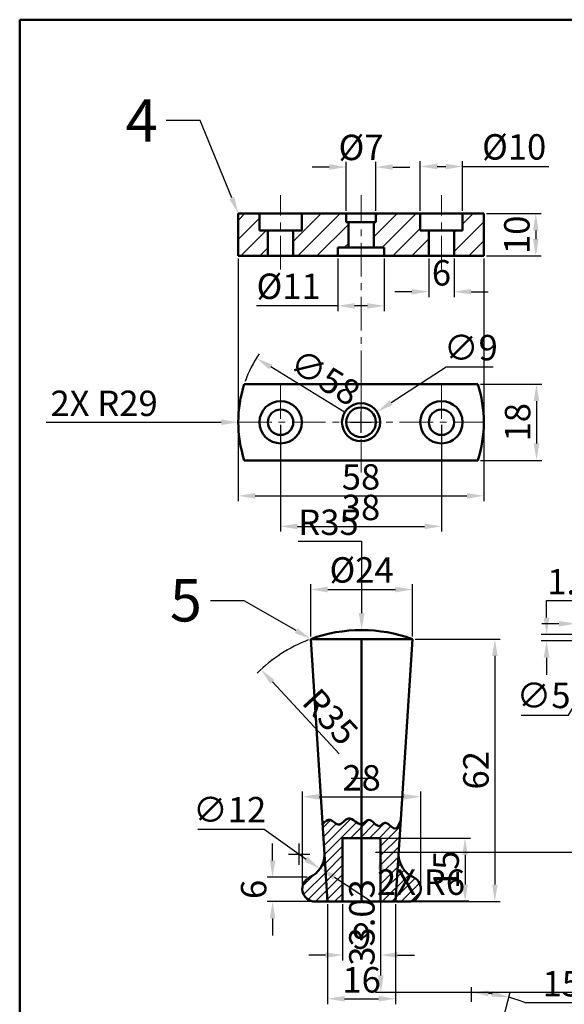
# Model space of a CAD drawing. Units: millimetres. Extents: x 1145 to 1687, y 12 to 400.
# Tile 2 of 6: x 1145 to 1274, y 168 to 400. Entities that reach past the tile are written whole.
import ezdxf
from ezdxf import colors
from ezdxf.entities.mleader import LeaderData, LeaderLine
from ezdxf.math import Vec2, Vec3

# ---------------------------------------------------------------- set-up
doc = ezdxf.new("R2010")
doc.units = ezdxf.units.MM
doc.header["$LTSCALE"] = 0.5
doc.linetypes.add('CENTER', pattern=[50.8, 31.75, -6.35, 6.35, -6.35])
for name, color, linetype, lineweight in [('M-CNTR', 1, 'CENTER', 18), ('M-DIMS', 2, 'Continuous', 25), ('M-HATC', 8, 'Continuous', 18), ('M-OUTL', 7, 'Continuous', 50), ('M-TEXT', 3, 'Continuous', 25)]:
    doc.layers.add(name, color=color, linetype=linetype, lineweight=lineweight)
doc.styles.get("Standard").update_dxf_attribs({"font": 'arial.ttf'})
doc.dimstyles.new('ISO-25', dxfattribs={"dimtxt": 6, "dimasz": 4, "dimexe": 1.25, "dimexo": 0.625, "dimtad": 1, "dimtoh": 1, "dimdec": 0, "dimtxsty": 'Standard', "dimcen": 2.5, "dimadec": 0, "dimazin": 0, "dimtfac": 1, "dimtdec": 0, "dimtofl": 0, "dimtmove": 0, "dimatfit": 3, "dimfxl": 1, "dimarcsym": 0})

# ---------------------------------------------------------------- blocks, each defined once
blk = doc.blocks.new('*D1')
at = {"layer": 'Defpoints', "color": 0, "ltscale": 0.5, "transparency": 16777216}
for p in [(1229.46, 365.34), (1222.46, 354.33), (1229.46, 354.33)]:
    blk.add_point(p, dxfattribs=at)
at = {"layer": 'M-DIMS', "color": 0, "lineweight": -2, "ltscale": 0.5, "transparency": 16777216}
for p, q in [((1218.46, 365.34), (1214.46, 365.34)), ((1222.46, 354.96), (1222.46, 366.59)), ((1229.46, 354.96), (1229.46, 366.59)), ((1233.46, 365.34), (1237.46, 365.34))]:
    blk.add_line(p, q, dxfattribs=at)
at = {"layer": 'M-DIMS', "color": 0, "ltscale": 0.5, "transparency": 16777216}
for points in [[(1218.46, 366), (1218.46, 364.67), (1222.46, 365.34)], [(1233.46, 366), (1233.46, 364.67), (1229.46, 365.34)]]:
    blk.add_solid(points, dxfattribs=at)
at = {"layer": 'M-DIMS', "color": 0, "ltscale": 0.5, "transparency": 16777216, "insert": (1225.96, 369.19), "char_height": 6, "attachment_point": 5}
blk.add_mtext('%%C7', dxfattribs=at)
blk = doc.blocks.new('*D2')
at = {"layer": 'Defpoints', "color": 0, "ltscale": 0.5, "transparency": 16777216}
for p in [(1249.96, 365.46), (1239.96, 354.33), (1249.96, 354.33)]:
    blk.add_point(p, dxfattribs=at)
at = {"layer": 'M-DIMS', "color": 0, "lineweight": -2, "ltscale": 0.5, "transparency": 16777216}
for p, q in [((1239.96, 354.96), (1239.96, 366.71)), ((1243.96, 365.46), (1245.96, 365.46)), ((1249.96, 354.96), (1249.96, 366.71)), ((1249.96, 365.46), (1270.32, 365.46))]:
    blk.add_line(p, q, dxfattribs=at)
at = {"layer": 'M-DIMS', "color": 0, "ltscale": 0.5, "transparency": 16777216}
for points in [[(1243.96, 366.13), (1243.96, 364.8), (1239.96, 365.46)], [(1245.96, 366.13), (1245.96, 364.8), (1249.96, 365.46)]]:
    blk.add_solid(points, dxfattribs=at)
at = {"layer": 'M-DIMS', "color": 0, "ltscale": 0.5, "transparency": 16777216, "insert": (1262.14, 369.32), "char_height": 6, "attachment_point": 5}
blk.add_mtext('%%C10', dxfattribs=at)
blk = doc.blocks.new('*D3')
at = {"layer": 'Defpoints', "color": 0, "ltscale": 0.5, "transparency": 16777216}
for p in [(1254.96, 354.33), (1254.96, 344.33), (1267.24, 344.33)]:
    blk.add_point(p, dxfattribs=at)
at = {"layer": 'M-DIMS', "color": 0, "lineweight": -2, "ltscale": 0.5, "transparency": 16777216}
for p, q in [((1255.59, 354.33), (1268.49, 354.33)), ((1267.24, 350.33), (1267.24, 348.33)), ((1255.59, 344.33), (1268.49, 344.33))]:
    blk.add_line(p, q, dxfattribs=at)
at = {"layer": 'M-DIMS', "color": 0, "ltscale": 0.5, "transparency": 16777216}
for points in [[(1266.58, 350.33), (1267.91, 350.33), (1267.24, 354.33)], [(1266.58, 348.33), (1267.91, 348.33), (1267.24, 344.33)]]:
    blk.add_solid(points, dxfattribs=at)
at = {"layer": 'M-DIMS', "color": 0, "ltscale": 0.5, "transparency": 16777216, "insert": (1263.55, 349.33), "char_height": 6, "attachment_point": 5, "rotation": 90}
blk.add_mtext('10', dxfattribs=at)
blk = doc.blocks.new('*D4')
at = {"layer": 'Defpoints', "color": 0, "ltscale": 0.5, "transparency": 16777216}
for p in [(1241.96, 344.33), (1247.96, 344.33), (1247.96, 335.89)]:
    blk.add_point(p, dxfattribs=at)
at = {"layer": 'M-DIMS', "color": 0, "lineweight": -2, "ltscale": 0.5, "transparency": 16777216}
for p, q in [((1241.96, 343.71), (1241.96, 334.64)), ((1247.96, 343.71), (1247.96, 334.64)), ((1237.96, 335.89), (1233.96, 335.89)), ((1251.96, 335.89), (1255.96, 335.89))]:
    blk.add_line(p, q, dxfattribs=at)
at = {"layer": 'M-DIMS', "color": 0, "ltscale": 0.5, "transparency": 16777216}
for points in [[(1237.96, 336.55), (1237.96, 335.22), (1241.96, 335.89)], [(1251.96, 336.55), (1251.96, 335.22), (1247.96, 335.89)]]:
    blk.add_solid(points, dxfattribs=at)
at = {"layer": 'M-DIMS', "color": 0, "ltscale": 0.5, "transparency": 16777216, "insert": (1244.96, 339.58), "char_height": 6, "attachment_point": 5}
blk.add_mtext('6', dxfattribs=at)
blk = doc.blocks.new('*D5')
at = {"layer": 'Defpoints', "color": 0, "ltscale": 0.5, "transparency": 16777216}
for p in [(1220.46, 344.33), (1231.46, 344.33), (1231.46, 332.54)]:
    blk.add_point(p, dxfattribs=at)
at = {"layer": 'M-DIMS', "color": 0, "lineweight": -2, "ltscale": 0.5, "transparency": 16777216}
for p, q in [((1220.46, 343.71), (1220.46, 331.29)), ((1231.46, 343.71), (1231.46, 331.29)), ((1220.46, 332.54), (1201.25, 332.54)), ((1227.46, 332.54), (1224.46, 332.54))]:
    blk.add_line(p, q, dxfattribs=at)
at = {"layer": 'M-DIMS', "color": 0, "ltscale": 0.5, "transparency": 16777216}
for points in [[(1224.46, 333.21), (1224.46, 331.87), (1220.46, 332.54)], [(1227.46, 333.21), (1227.46, 331.87), (1231.46, 332.54)]]:
    blk.add_solid(points, dxfattribs=at)
at = {"layer": 'M-DIMS', "color": 0, "ltscale": 0.5, "transparency": 16777216, "insert": (1208.86, 336.4), "char_height": 6, "attachment_point": 5}
blk.add_mtext('%%C11', dxfattribs=at)
blk = doc.blocks.new('*D6')
at = {"layer": 'Defpoints', "color": 0, "ltscale": 0.5, "transparency": 16777216}
for p in [(1206.96, 305.06), (1244.96, 305.06), (1244.96, 280.47)]:
    blk.add_point(p, dxfattribs=at)
at = {"layer": 'M-DIMS', "color": 0, "lineweight": -2, "ltscale": 0.5, "transparency": 16777216}
for p, q in [((1206.96, 304.44), (1206.96, 279.22)), ((1244.96, 304.44), (1244.96, 279.22)), ((1210.96, 280.47), (1240.96, 280.47))]:
    blk.add_line(p, q, dxfattribs=at)
at = {"layer": 'M-DIMS', "color": 0, "ltscale": 0.5, "transparency": 16777216}
for points in [[(1210.96, 281.14), (1210.96, 279.8), (1206.96, 280.47)], [(1240.96, 281.14), (1240.96, 279.8), (1244.96, 280.47)]]:
    blk.add_solid(points, dxfattribs=at)
at = {"layer": 'M-DIMS', "color": 0, "ltscale": 0.5, "transparency": 16777216, "insert": (1225.96, 284.16), "char_height": 6, "attachment_point": 5}
blk.add_mtext('38', dxfattribs=at)
blk = doc.blocks.new('*D7')
at = {"layer": 'Defpoints', "color": 0, "ltscale": 0.5, "transparency": 16777216}
for p in [(1253.53, 314.06), (1253.53, 296.06), (1267.41, 296.06)]:
    blk.add_point(p, dxfattribs=at)
at = {"layer": 'M-DIMS', "color": 0, "lineweight": -2, "ltscale": 0.5, "transparency": 16777216}
for p, q in [((1254.16, 314.06), (1268.66, 314.06)), ((1267.41, 310.06), (1267.41, 300.06)), ((1254.16, 296.06), (1268.66, 296.06))]:
    blk.add_line(p, q, dxfattribs=at)
at = {"layer": 'M-DIMS', "color": 0, "ltscale": 0.5, "transparency": 16777216}
for points in [[(1266.74, 310.06), (1268.07, 310.06), (1267.41, 314.06)], [(1266.74, 300.06), (1268.07, 300.06), (1267.41, 296.06)]]:
    blk.add_solid(points, dxfattribs=at)
at = {"layer": 'M-DIMS', "color": 0, "ltscale": 0.5, "transparency": 16777216, "insert": (1263.72, 305.06), "char_height": 6, "attachment_point": 5, "rotation": 90}
blk.add_mtext('18', dxfattribs=at)
blk = doc.blocks.new('*D8')
at = {"layer": 'Defpoints', "color": 0, "ltscale": 0.5, "transparency": 16777216}
for p in [(1229.74, 307.51), (1222.19, 302.62)]:
    blk.add_point(p, dxfattribs=at)
at = {"layer": 'M-DIMS', "color": 0, "lineweight": -2, "ltscale": 0.5, "transparency": 16777216}
for p, q in [((1246.05, 318.06), (1233.1, 309.68)), ((1257.14, 318.06), (1246.05, 318.06)), ((1225.96, 302.56), (1225.96, 307.56)), ((1223.46, 305.06), (1228.46, 305.06))]:
    blk.add_line(p, q, dxfattribs=at)
at = {"layer": 'M-DIMS', "color": 0, "ltscale": 0.5, "transparency": 16777216}
blk.add_solid([(1232.74, 310.24), (1233.46, 309.12), (1229.74, 307.51)], dxfattribs=at)
at = {"layer": 'M-DIMS', "color": 0, "ltscale": 0.5, "transparency": 16777216, "insert": (1251.91, 321.91), "char_height": 6, "attachment_point": 5}
blk.add_mtext('∅9', dxfattribs=at)
blk = doc.blocks.new('*D26')
at = {"layer": 'Defpoints', "color": 0, "ltscale": 0.5, "transparency": 16777216}
for p in [(1221.6, 191.85), (1230.6, 191.85), (1230.6, 179.21)]:
    blk.add_point(p, dxfattribs=at)
at = {"layer": 'M-DIMS', "color": 0, "lineweight": -2, "ltscale": 0.5, "transparency": 16777216}
for p, q in [((1221.6, 191.22), (1221.6, 177.96)), ((1230.6, 191.22), (1230.6, 177.96)), ((1217.6, 179.21), (1213.6, 179.21)), ((1234.6, 179.21), (1238.6, 179.21))]:
    blk.add_line(p, q, dxfattribs=at)
at = {"layer": 'M-DIMS', "color": 0, "ltscale": 0.5, "transparency": 16777216}
for points in [[(1217.6, 179.87), (1217.6, 178.54), (1221.6, 179.21)], [(1234.6, 179.87), (1234.6, 178.54), (1230.6, 179.21)]]:
    blk.add_solid(points, dxfattribs=at)
at = {"layer": 'M-DIMS', "color": 0, "ltscale": 0.5, "transparency": 16777216, "insert": (1226.1, 182.9), "char_height": 6, "attachment_point": 5}
blk.add_mtext('9', dxfattribs=at)
blk = doc.blocks.new('*D27')
at = {"layer": 'Defpoints', "color": 0, "ltscale": 0.5, "transparency": 16777216}
for p in [(1218.07, 191.85), (1234.12, 191.85), (1234.12, 168.89)]:
    blk.add_point(p, dxfattribs=at)
at = {"layer": 'M-DIMS', "color": 0, "lineweight": -2, "ltscale": 0.5, "transparency": 16777216}
for p, q in [((1218.07, 191.22), (1218.07, 167.64)), ((1234.12, 191.22), (1234.12, 167.64)), ((1222.07, 168.89), (1230.12, 168.89))]:
    blk.add_line(p, q, dxfattribs=at)
at = {"layer": 'M-DIMS', "color": 0, "ltscale": 0.5, "transparency": 16777216}
for points in [[(1222.07, 169.55), (1222.07, 168.22), (1218.07, 168.89)], [(1230.12, 169.55), (1230.12, 168.22), (1234.12, 168.89)]]:
    blk.add_solid(points, dxfattribs=at)
at = {"layer": 'M-DIMS', "color": 0, "ltscale": 0.5, "transparency": 16777216, "insert": (1226.1, 172.58), "char_height": 6, "attachment_point": 5}
blk.add_mtext('16', dxfattribs=at)
blk = doc.blocks.new('*D28')
at = {"layer": 'Defpoints', "color": 0, "ltscale": 0.5, "transparency": 16777216}
for p in [(1238.1, 253.85), (1234.12, 191.85), (1257.57, 191.85)]:
    blk.add_point(p, dxfattribs=at)
at = {"layer": 'M-DIMS', "color": 0, "lineweight": -2, "ltscale": 0.5, "transparency": 16777216}
for p, q in [((1238.72, 253.85), (1258.82, 253.85)), ((1257.57, 249.85), (1257.57, 195.85)), ((1234.75, 191.85), (1258.82, 191.85))]:
    blk.add_line(p, q, dxfattribs=at)
at = {"layer": 'M-DIMS', "color": 0, "ltscale": 0.5, "transparency": 16777216}
for points in [[(1256.91, 249.85), (1258.24, 249.85), (1257.57, 253.85)], [(1256.91, 195.85), (1258.24, 195.85), (1257.57, 191.85)]]:
    blk.add_solid(points, dxfattribs=at)
at = {"layer": 'M-DIMS', "color": 0, "ltscale": 0.5, "transparency": 16777216, "insert": (1253.88, 222.85), "char_height": 6, "attachment_point": 5, "rotation": 90}
blk.add_mtext('62', dxfattribs=at)
blk = doc.blocks.new('*D29')
at = {"layer": 'Defpoints', "color": 0, "ltscale": 0.5, "transparency": 16777216}
for p in [(1226.1, 206.85), (1226.1, 191.85), (1250.54, 191.85)]:
    blk.add_point(p, dxfattribs=at)
at = {"layer": 'M-DIMS', "color": 0, "lineweight": -2, "ltscale": 0.5, "transparency": 16777216}
for p, q in [((1226.72, 206.85), (1251.79, 206.85)), ((1250.54, 202.85), (1250.54, 195.85)), ((1226.72, 191.85), (1251.79, 191.85))]:
    blk.add_line(p, q, dxfattribs=at)
at = {"layer": 'M-DIMS', "color": 0, "ltscale": 0.5, "transparency": 16777216}
for points in [[(1249.87, 202.85), (1251.2, 202.85), (1250.54, 206.85)], [(1249.87, 195.85), (1251.2, 195.85), (1250.54, 191.85)]]:
    blk.add_solid(points, dxfattribs=at)
at = {"layer": 'M-DIMS', "color": 0, "ltscale": 0.5, "transparency": 16777216, "insert": (1246.85, 199.35), "char_height": 6, "attachment_point": 5, "rotation": 90}
blk.add_mtext('15', dxfattribs=at)
blk = doc.blocks.new('*D30')
at = {"layer": 'Defpoints', "color": 0, "ltscale": 0.5, "transparency": 16777216}
for p in [(1205.07, 197.58), (1213.85, 197.58), (1215.1, 191.85)]:
    blk.add_point(p, dxfattribs=at)
at = {"layer": 'M-DIMS', "color": 0, "lineweight": -2, "ltscale": 0.5, "transparency": 16777216}
for p, q in [((1205.07, 201.58), (1205.07, 205.58)), ((1213.23, 197.58), (1203.82, 197.58)), ((1214.47, 191.85), (1203.82, 191.85)), ((1205.07, 187.85), (1205.07, 183.85))]:
    blk.add_line(p, q, dxfattribs=at)
at = {"layer": 'M-DIMS', "color": 0, "ltscale": 0.5, "transparency": 16777216}
for points in [[(1204.41, 201.58), (1205.74, 201.58), (1205.07, 197.58)], [(1204.41, 187.85), (1205.74, 187.85), (1205.07, 191.85)]]:
    blk.add_solid(points, dxfattribs=at)
at = {"layer": 'M-DIMS', "color": 0, "ltscale": 0.5, "transparency": 16777216, "insert": (1201.38, 194.71), "char_height": 6, "attachment_point": 5, "rotation": 90}
blk.add_mtext('6', dxfattribs=at)
blk = doc.blocks.new('*D31')
at = {"layer": 'Defpoints', "color": 0, "ltscale": 0.5, "transparency": 16777216}
for p in [(1206.47, 206.51), (1216.25, 199.56)]:
    blk.add_point(p, dxfattribs=at)
at = {"layer": 'M-DIMS', "color": 0, "lineweight": -2, "ltscale": 0.5, "transparency": 16777216}
for p, q in [((1187.4, 208.92), (1203.08, 208.92)), ((1203.08, 208.92), (1212.99, 201.88))]:
    blk.add_line(p, q, dxfattribs=at)
at = {"layer": 'M-DIMS', "color": 0, "ltscale": 0.5, "transparency": 16777216}
blk.add_solid([(1213.38, 202.42), (1212.61, 201.33), (1216.25, 199.56)], dxfattribs=at)
at = {"layer": 'M-DIMS', "color": 0, "ltscale": 0.5, "transparency": 16777216, "insert": (1194.93, 212.77), "char_height": 6, "attachment_point": 5}
blk.add_mtext('∅12', dxfattribs=at)
blk = doc.blocks.new('*D32')
at = {"layer": 'Defpoints', "color": 0, "ltscale": 0.5, "transparency": 16777216}
for p in [(1238.1, 265.55), (1214.1, 253.85), (1238.1, 253.85)]:
    blk.add_point(p, dxfattribs=at)
at = {"layer": 'M-DIMS', "color": 0, "lineweight": -2, "ltscale": 0.5, "transparency": 16777216}
for p, q in [((1214.1, 254.47), (1214.1, 266.8)), ((1218.1, 265.55), (1234.1, 265.55)), ((1238.1, 254.47), (1238.1, 266.8))]:
    blk.add_line(p, q, dxfattribs=at)
at = {"layer": 'M-DIMS', "color": 0, "ltscale": 0.5, "transparency": 16777216}
for points in [[(1218.1, 266.21), (1218.1, 264.88), (1214.1, 265.55)], [(1234.1, 266.21), (1234.1, 264.88), (1238.1, 265.55)]]:
    blk.add_solid(points, dxfattribs=at)
at = {"layer": 'M-DIMS', "color": 0, "ltscale": 0.5, "transparency": 16777216, "insert": (1226.1, 269.4), "char_height": 6, "attachment_point": 5}
blk.add_mtext('%%C24', dxfattribs=at)
blk = doc.blocks.new('*D34')
at = {"layer": 'Defpoints', "color": 0, "ltscale": 0.5, "transparency": 16777216}
for p in [(1283.69, 257.48), (1276.69, 249.68), (1283.69, 250.43)]:
    blk.add_point(p, dxfattribs=at)
at = {"layer": 'M-DIMS', "color": 0, "lineweight": -2, "ltscale": 0.5, "transparency": 16777216}
for p, q in [((1276.69, 250.31), (1276.69, 258.73)), ((1283.69, 251.06), (1283.69, 258.73)), ((1272.69, 257.48), (1268.69, 257.48)), ((1287.69, 257.48), (1291.69, 257.48))]:
    blk.add_line(p, q, dxfattribs=at)
at = {"layer": 'M-DIMS', "color": 0, "ltscale": 0.5, "transparency": 16777216}
for points in [[(1272.69, 258.14), (1272.69, 256.81), (1276.69, 257.48)], [(1287.69, 258.14), (1287.69, 256.81), (1283.69, 257.48)]]:
    blk.add_solid(points, dxfattribs=at)
at = {"layer": 'M-DIMS', "color": 0, "ltscale": 0.5, "transparency": 16777216, "insert": (1280.19, 261.1), "char_height": 6, "attachment_point": 5}
blk.add_mtext('7', dxfattribs=at)
blk = doc.blocks.new('*D40')
at = {"layer": 'Defpoints', "color": 0, "ltscale": 0.5, "transparency": 16777216}
for p in [(1284.98, 252.57), (1282.4, 248.29)]:
    blk.add_point(p, dxfattribs=at)
at = {"layer": 'M-DIMS', "color": 0, "lineweight": -2, "ltscale": 0.5, "transparency": 16777216}
for p, q in [((1283.69, 247.93), (1283.69, 252.93)), ((1281.19, 250.43), (1286.19, 250.43)), ((1274.96, 235.89), (1280.34, 244.86)), ((1263.83, 235.89), (1274.96, 235.89))]:
    blk.add_line(p, q, dxfattribs=at)
at = {"layer": 'M-DIMS', "color": 0, "ltscale": 0.5, "transparency": 16777216}
blk.add_solid([(1279.77, 245.2), (1280.91, 244.52), (1282.4, 248.29)], dxfattribs=at)
at = {"layer": 'M-DIMS', "color": 0, "ltscale": 0.5, "transparency": 16777216, "insert": (1269.08, 239.75), "char_height": 6, "attachment_point": 5}
blk.add_mtext('∅5', dxfattribs=at)
blk = doc.blocks.new('*D53')
at = {"layer": 'Defpoints', "color": 0, "ltscale": 0.5, "transparency": 16777216}
for p in [(1201.23, 320.2), (1250.7, 289.92)]:
    blk.add_point(p, dxfattribs=at)
at = {"layer": 'M-DIMS', "color": 0, "lineweight": -2, "ltscale": 0.5, "transparency": 16777216}
blk.add_line((1222.03, 307.47), (1204.64, 318.11), dxfattribs=at)
blk.add_arc((1225.96, 305.06), 29, 146.0564, 160.6852, dxfattribs=at)
at = {"layer": 'M-DIMS', "color": 0, "ltscale": 0.5, "transparency": 16777216}
blk.add_solid([(1204.99, 318.68), (1204.29, 317.54), (1201.23, 320.2)], dxfattribs=at)
at = {"layer": 'M-DIMS', "color": 0, "ltscale": 0.5, "transparency": 16777216, "insert": (1217.06, 315.04), "char_height": 6, "attachment_point": 5, "rotation": 328.526}
blk.add_mtext('∅58', dxfattribs=at)
blk = doc.blocks.new('*D54')
at = {"layer": 'Defpoints', "color": 0, "ltscale": 0.5, "transparency": 16777216}
for p in [(1202.32, 246.65), (1226.1, 220.97)]:
    blk.add_point(p, dxfattribs=at)
at = {"layer": 'M-DIMS', "color": 0, "lineweight": -2, "ltscale": 0.5, "transparency": 16777216}
blk.add_line((1220.78, 226.71), (1205.04, 243.72), dxfattribs=at)
blk.add_arc((1226.1, 220.97), 35, 111.0742, 134.8421, dxfattribs=at)
at = {"layer": 'M-DIMS', "color": 0, "ltscale": 0.5, "transparency": 16777216}
blk.add_solid([(1205.52, 244.17), (1204.55, 243.26), (1202.32, 246.65)], dxfattribs=at)
at = {"layer": 'M-DIMS', "color": 0, "ltscale": 0.5, "transparency": 16777216, "insert": (1218.18, 234.96), "char_height": 6, "attachment_point": 5, "rotation": 312.7958}
blk.add_mtext('R35', dxfattribs=at)
blk = doc.blocks.new('*D55')
at = {"layer": 'Defpoints', "color": 0, "ltscale": 0.5, "transparency": 16777216}
for p in [(1240.1, 216.6), (1212.11, 195.12), (1240.1, 194.81)]:
    blk.add_point(p, dxfattribs=at)
at = {"layer": 'M-DIMS', "color": 0, "lineweight": -2, "ltscale": 0.5, "transparency": 16777216}
for p, q in [((1212.11, 195.74), (1212.11, 217.85)), ((1216.11, 216.6), (1236.1, 216.6)), ((1240.1, 195.44), (1240.1, 217.85))]:
    blk.add_line(p, q, dxfattribs=at)
at = {"layer": 'M-DIMS', "color": 0, "ltscale": 0.5, "transparency": 16777216}
for points in [[(1216.11, 217.27), (1216.11, 215.93), (1212.11, 216.6)], [(1236.1, 217.27), (1236.1, 215.93), (1240.1, 216.6)]]:
    blk.add_solid(points, dxfattribs=at)
at = {"layer": 'M-DIMS', "color": 0, "ltscale": 0.5, "transparency": 16777216, "insert": (1226.1, 220.29), "char_height": 6, "attachment_point": 5}
blk.add_mtext('28', dxfattribs=at)
blk = doc.blocks.new('*D73')
at = {"layer": 'Defpoints', "color": 0, "ltscale": 0.5, "transparency": 16777216}
for p in [(1255.04, 170.27), (1252.07, 167.52), (1257.42, 156.31), (1252.07, 136.31), (1252.07, 136.31)]:
    blk.add_point(p, dxfattribs=at)
at = {"layer": 'M-DIMS', "color": 0, "lineweight": -2, "ltscale": 0.5, "transparency": 16777216}
for p, q in [((1252.07, 168.14), (1252.07, 171.65)), ((1257.59, 156.91), (1261.21, 170.44)), ((1264.68, 167.98), (1281.14, 167.98))]:
    blk.add_line(p, q, dxfattribs=at)
for start, end in [(81.7274, 83.2726), (68.2726, 75)]:
    blk.add_arc((1252.07, 136.31), 34.09, start, end, dxfattribs=at)
at = {"layer": 'M-DIMS', "color": 0, "ltscale": 0.5, "transparency": 16777216}
for points in [[(1256.02, 169.5), (1256.1, 170.83), (1252.07, 170.4)], [(1257.1, 170.69), (1256.84, 169.39), (1260.89, 169.24)]]:
    blk.add_solid(points, dxfattribs=at)
at = {"layer": 'M-DIMS', "color": 0, "ltscale": 0.5, "transparency": 16777216, "insert": (1274.91, 171.66), "char_height": 6, "attachment_point": 5}
blk.add_mtext('15°', dxfattribs=at)
blk = doc.blocks.new('*D89')
at = {"layer": 'Defpoints', "color": 0, "ltscale": 0.5, "transparency": 16777216}
for p in [(1196.96, 344.33), (1254.96, 344.33), (1254.96, 287.68)]:
    blk.add_point(p, dxfattribs=at)
at = {"layer": 'M-DIMS', "color": 0, "lineweight": -2, "ltscale": 0.5, "transparency": 16777216}
for p, q in [((1196.96, 343.71), (1196.96, 286.43)), ((1254.96, 343.71), (1254.96, 286.43)), ((1200.96, 287.68), (1250.96, 287.68))]:
    blk.add_line(p, q, dxfattribs=at)
at = {"layer": 'M-DIMS', "color": 0, "ltscale": 0.5, "transparency": 16777216}
for points in [[(1200.96, 288.34), (1200.96, 287.01), (1196.96, 287.68)], [(1250.96, 288.34), (1250.96, 287.01), (1254.96, 287.68)]]:
    blk.add_solid(points, dxfattribs=at)
at = {"layer": 'M-DIMS', "color": 0, "ltscale": 0.5, "transparency": 16777216, "insert": (1225.96, 291.37), "char_height": 6, "attachment_point": 5}
blk.add_mtext('58', dxfattribs=at)
blk = doc.blocks.new('*D100')
at = {"layer": 'Defpoints', "color": 0, "ltscale": 0.5, "transparency": 16777216}
for p in [(1230.63, 203.42), (1359.03, 203.42), (1359.03, 170.39)]:
    blk.add_point(p, dxfattribs=at)
at = {"layer": 'M-DIMS', "color": 0, "lineweight": -2, "ltscale": 0.5, "transparency": 16777216}
for p, q in [((1358.41, 203.42), (1229.38, 203.42)), ((1230.63, 174.39), (1230.63, 199.42)), ((1358.41, 170.39), (1229.38, 170.39))]:
    blk.add_line(p, q, dxfattribs=at)
at = {"layer": 'M-DIMS', "color": 0, "ltscale": 0.5, "transparency": 16777216}
for points in [[(1229.96, 199.42), (1231.29, 199.42), (1230.63, 203.42)], [(1229.96, 174.39), (1231.29, 174.39), (1230.63, 170.39)]]:
    blk.add_solid(points, dxfattribs=at)
at = {"layer": 'M-DIMS', "color": 0, "ltscale": 0.5, "transparency": 16777216, "insert": (1226.94, 186.91), "char_height": 6, "attachment_point": 5, "rotation": 90}
blk.add_mtext('33.03', dxfattribs=at)
blk = doc.blocks.new('*D101')
at = {"layer": 'Defpoints', "color": 0, "ltscale": 0.5, "transparency": 16777216}
for p in [(1269.79, 254.93), (1278.19, 254.93), (1276.69, 253.43)]:
    blk.add_point(p, dxfattribs=at)
at = {"layer": 'M-DIMS', "color": 0, "lineweight": -2, "ltscale": 0.5, "transparency": 16777216}
for p, q in [((1269.79, 258.93), (1269.79, 262.93)), ((1269.79, 262.93), (1280.82, 262.93)), ((1277.56, 254.93), (1268.54, 254.93)), ((1276.06, 253.43), (1268.54, 253.43)), ((1269.79, 249.43), (1269.79, 245.43))]:
    blk.add_line(p, q, dxfattribs=at)
at = {"layer": 'M-DIMS', "color": 0, "ltscale": 0.5, "transparency": 16777216}
for points in [[(1269.12, 258.93), (1270.46, 258.93), (1269.79, 254.93)], [(1269.12, 249.43), (1270.46, 249.43), (1269.79, 253.43)]]:
    blk.add_solid(points, dxfattribs=at)
at = {"layer": 'M-DIMS', "color": 0, "ltscale": 0.5, "transparency": 16777216, "insert": (1275.62, 266.62), "char_height": 6, "attachment_point": 5}
blk.add_mtext('1.5', dxfattribs=at)
blk = doc.blocks.new('*D112')
at = {"layer": 'Defpoints', "color": 0, "ltscale": 0.5, "transparency": 16777216}
for p in [(1196.96, 305.06), (1225.96, 305.06)]:
    blk.add_point(p, dxfattribs=at)
at = {"layer": 'M-DIMS', "color": 0, "lineweight": -2, "ltscale": 0.5, "transparency": 16777216}
for p, q in [((1225.96, 302.56), (1225.96, 307.56)), ((1151.6, 305.06), (1179.56, 305.06)), ((1179.56, 305.06), (1192.96, 305.06)), ((1223.46, 305.06), (1228.46, 305.06))]:
    blk.add_line(p, q, dxfattribs=at)
at = {"layer": 'M-DIMS', "color": 0, "ltscale": 0.5, "transparency": 16777216}
blk.add_solid([(1192.96, 305.73), (1192.96, 304.39), (1196.96, 305.06)], dxfattribs=at)
at = {"layer": 'M-DIMS', "color": 0, "ltscale": 0.5, "transparency": 16777216, "insert": (1165.27, 308.75), "char_height": 6, "attachment_point": 5}
blk.add_mtext('2X R29', dxfattribs=at)
blk = doc.blocks.new('*D113')
at = {"layer": 'Defpoints', "color": 0, "ltscale": 0.5, "transparency": 16777216}
for p in [(1226.1, 255.97), (1226.1, 220.97)]:
    blk.add_point(p, dxfattribs=at)
at = {"layer": 'M-DIMS', "color": 0, "lineweight": -2, "ltscale": 0.5, "transparency": 16777216}
for p, q in [((1211.09, 276.97), (1226.1, 276.97)), ((1226.1, 276.97), (1226.1, 259.97)), ((1226.1, 218.47), (1226.1, 223.47)), ((1223.6, 220.97), (1228.6, 220.97))]:
    blk.add_line(p, q, dxfattribs=at)
at = {"layer": 'M-DIMS', "color": 0, "ltscale": 0.5, "transparency": 16777216}
blk.add_solid([(1226.76, 259.97), (1225.43, 259.97), (1226.1, 255.97)], dxfattribs=at)
at = {"layer": 'M-DIMS', "color": 0, "ltscale": 0.5, "transparency": 16777216, "insert": (1218.28, 280.66), "char_height": 6, "attachment_point": 5}
blk.add_mtext('R35', dxfattribs=at)
blk = doc.blocks.new('*D114')
at = {"layer": 'Defpoints', "color": 0, "ltscale": 0.5, "transparency": 16777216}
for p in [(1211.36, 203.04), (1216.37, 199.73)]:
    blk.add_point(p, dxfattribs=at)
at = {"layer": 'M-DIMS', "color": 0, "lineweight": -2, "ltscale": 0.5, "transparency": 16777216}
for p, q in [((1211.36, 200.54), (1211.36, 205.54)), ((1208.86, 203.04), (1213.86, 203.04)), ((1228.17, 191.96), (1219.71, 197.53)), ((1251.46, 191.96), (1228.17, 191.96))]:
    blk.add_line(p, q, dxfattribs=at)
at = {"layer": 'M-DIMS', "color": 0, "ltscale": 0.5, "transparency": 16777216}
blk.add_solid([(1220.08, 198.09), (1219.35, 196.98), (1216.37, 199.73)], dxfattribs=at)
at = {"layer": 'M-DIMS', "color": 0, "ltscale": 0.5, "transparency": 16777216, "insert": (1240.13, 195.65), "char_height": 6, "attachment_point": 5}
blk.add_mtext('2X R6', dxfattribs=at)

msp = doc.modelspace()

# ---------------------------------------------------------------- hatches: boundary and pattern name
at = {"layer": 'M-HATC', "ltscale": 0.5}
h = msp.add_hatch(dxfattribs=at)
h.set_pattern_fill('ANSI31', color=256)
h.set_pattern_definition([(45, (519.2703, 155.495), (-2.245064, 2.245064), [])])
h.paths.add_polyline_path([(1203.9648, 350.3344), (1201.9648, 350.3344), (1201.9648, 354.3344), (1196.9648, 354.3344), (1196.9648, 344.3344), (1203.9648, 344.3344)])
h.paths.add_polyline_path([(1220.4648, 346.3344), (1222.9648, 346.3344), (1222.9648, 352.3344), (1222.4648, 352.3344), (1222.4648, 354.3344), (1211.9648, 354.3344), (1211.9648, 350.3344), (1209.9648, 350.3344), (1209.9648, 344.3344), (1220.4648, 344.3344)])
h.paths.add_polyline_path([(1241.9648, 344.3344), (1241.9648, 350.3344), (1239.9648, 350.3344), (1239.9648, 354.3344), (1229.4648, 354.3344), (1229.4648, 352.3344), (1228.9648, 352.3344), (1228.9648, 346.3344), (1231.4648, 346.3344), (1231.4648, 344.3344)])
h.paths.add_polyline_path([(1254.9648, 354.3344), (1249.9648, 354.3344), (1249.9648, 350.3344), (1247.9648, 350.3344), (1247.9648, 344.3344), (1254.9648, 344.3344)])
h = msp.add_hatch(dxfattribs=at)
h.set_pattern_fill('ANSI31', color=256, scale=0.5)
h.set_pattern_definition([(45, (309.0715, 64.712), (-1.122532, 1.122532), [])])
edge = h.paths.add_edge_path()
edge.add_line((1221.5962, 206.8469), (1226.0962, 206.8469))
edge.add_line((1226.0962, 206.8469), (1226.0962, 210.1606))
edge.add_spline(control_points=[(1226.0962, 210.1606), (1225.1115, 209.9151), (1223.1238, 212.9907), (1220.7699, 208.8784), (1218.7113, 211.8853), (1217.4899, 210.7128), (1216.9146, 210.1605)], knot_values=[0, 0, 0, 0, 3.31304986, 6.16040245, 8.40124344, 10.39663985, 10.39663985, 10.39663985, 10.39663985], degree=3, periodic=0)
edge.add_line((1216.8964, 210.1431), (1218.0687, 191.8469))
edge.add_line((1218.0687, 191.8469), (1221.5962, 191.8469))
edge.add_line((1221.5962, 191.8469), (1221.5962, 206.8469))
h.paths.add_polyline_path([(1217.3603, 202.9025, -0.28775426), (1213.8514, 197.5765, 0.80607302), (1215.0962, 191.8469), (1218.0687, 191.8469)])
h.paths.add_polyline_path([(1238.3409, 197.5765, -0.28775426), (1234.832, 202.9025), (1234.1236, 191.8469), (1237.0962, 191.8469, 0.80607302)])
edge = h.paths.add_edge_path()
edge.add_spline(control_points=[(1235.3263, 210.9148), (1234.9058, 209.9628), (1233.9937, 207.8981), (1231.8911, 211.377), (1229.8896, 208.6771), (1228.0403, 212.2947), (1226.6755, 210.305), (1226.0962, 210.1606)], knot_values=[10.39663985, 10.39663985, 10.39663985, 10.39663985, 12.72069211, 15.43721405, 16.91039682, 19.79725618, 21.74648416, 21.74648416, 21.74648416, 21.74648416], degree=3, periodic=0)
edge.add_line((1226.0962, 210.1606), (1226.0962, 206.8469))
edge.add_line((1226.0962, 206.8469), (1230.5962, 206.8469))
edge.add_line((1230.5962, 206.8469), (1230.5962, 191.8469))
edge.add_line((1230.5962, 191.8469), (1234.1236, 191.8469))
edge.add_line((1234.1236, 191.8469), (1234.832, 202.9025))
edge.add_line((1234.832, 202.9025), (1235.3485, 210.9649))

# ---------------------------------------------------------------- linework, layer by layer
at = {"layer": 'M-CNTR', "ltscale": 0.5}
for p, q in [((1206.9648, 341.1579), (1206.9648, 358.7124)), ((1225.9648, 314.0602), (1225.9648, 358.7124)), ((1244.9648, 341.1579), (1244.9648, 358.7124)), ((1206.9648, 293.1766), (1206.9648, 314.0602)), ((1225.9648, 293.1766), (1225.9648, 314.0602)), ((1244.9648, 293.1766), (1244.9648, 314.0602)), ((1196.9648, 305.0602), (1254.9648, 305.0602))]:
    msp.add_line(p, q, dxfattribs=at)
at = {"layer": 'M-OUTL', "ltscale": 0.5}
for p, q in [((1196.9648, 344.3344), (1196.9648, 354.3344)), ((1196.9648, 354.3344), (1254.9648, 354.3344)), ((1201.9648, 350.3344), (1201.9648, 354.3344)), ((1211.9648, 350.3344), (1211.9648, 354.3344)), ((1222.4648, 352.3344), (1222.4648, 354.3344)), ((1229.4648, 352.3344), (1229.4648, 354.3344)), ((1239.9648, 350.3344), (1239.9648, 354.3344)), ((1249.9648, 350.3344), (1249.9648, 354.3344)), ((1254.9648, 354.3344), (1254.9648, 344.3344)), ((1222.4648, 352.3344), (1229.4648, 352.3344)), ((1222.9648, 346.3344), (1222.9648, 352.3344)), ((1228.9648, 346.3344), (1228.9648, 352.3344)), ((1201.9648, 350.3344), (1211.9648, 350.3344)), ((1203.9648, 344.3344), (1203.9648, 350.3344)), ((1209.9648, 344.3344), (1209.9648, 350.3344)), ((1249.9648, 350.3344), (1239.9648, 350.3344)), ((1241.9648, 344.3344), (1241.9648, 350.3344)), ((1247.9648, 344.3344), (1247.9648, 350.3344)), ((1196.9648, 344.3344), (1254.9648, 344.3344)), ((1220.4648, 344.3344), (1220.4648, 346.3344)), ((1220.4648, 346.3344), (1231.4648, 346.3344)), ((1231.4648, 344.3344), (1231.4648, 346.3344)), ((1198.3968, 314.0602), (1253.5329, 314.0602)), ((1198.3968, 296.0602), (1253.5329, 296.0602)), ((1214.0962, 253.8469), (1238.0962, 253.8469)), ((1218.0687, 191.8469), (1214.0962, 253.8469)), ((1226.0962, 191.8469), (1226.0962, 253.8469)), ((1234.1236, 191.8469), (1238.0962, 253.8469)), ((1221.5962, 206.8469), (1221.5962, 191.8469)), ((1221.5962, 206.8469), (1230.5962, 206.8469)), ((1230.5962, 191.8469), (1230.5962, 206.8469)), ((1212.0962, 197.8469), (1212.0962, 197.8469)), ((1215.0962, 191.8469), (1237.0962, 191.8469)), ((1221.5962, 191.8469), (1230.5962, 191.8469))]:
    msp.add_line(p, q, dxfattribs=at)
msp.add_lwpolyline([(1145.3327, 400.1417), (1687.1285, 400.1417), (1687.1285, 12.2645), (1145.3327, 12.2645)], close=True, dxfattribs=at)
for centre, radius in [((1206.9648, 305.0602), 5), ((1225.9648, 305.0602), 4.5), ((1244.9648, 305.0602), 5), ((1206.9648, 305.0602), 3), ((1225.9648, 305.0602), 3.5), ((1244.9648, 305.0602), 3)]:
    msp.add_circle(centre, radius, dxfattribs=at)
for centre, radius, start, end in [((1225.9648, 305.0602), 29, 161.919987, 198.080013), ((1225.9648, 305.0602), 29, 341.919987, 18.080013), ((1226.0962, 220.9684), 35, 69.948957, 110.051043), ((1211.3618, 203.0356), 6, 294.514598, 358.728192), ((1240.8305, 203.0356), 6, 181.271808, 245.485402), ((1215.0962, 194.8469), 3, 114.514598, 270), ((1237.0962, 194.8469), 3, 270, 65.485402)]:
    msp.add_arc(centre, radius, start, end, dxfattribs=at)
msp.add_open_spline([(1216.9146, 210.1605), (1217.4899, 210.7128), (1218.7113, 211.8853), (1220.7699, 208.8784), (1223.1238, 212.9907), (1225.7405, 208.942), (1228.0403, 212.2947), (1229.8896, 208.6771), (1231.8911, 211.377), (1233.9937, 207.8981), (1234.9058, 209.9628), (1235.3263, 210.9148)], degree=3, knots=[0, 0, 0, 0, 1.99539641, 4.2362374, 7.08358999, 10.39663985, 12.34586782, 15.23272719, 16.70590995, 19.42243189, 21.74648416, 21.74648416, 21.74648416, 21.74648416], dxfattribs=at)

# ---------------------------------------------------------------- dimensions: what is measured, and where the dimension line sits
at = {"layer": 'M-DIMS', "ltscale": 0.5}
for base, p1, p2, text, picture, middle in [((1229.4648, 365.3374), (1222.4648, 354.3344), (1229.4648, 354.3344), '%%C7', '*D1', (1225.9648, 365.3374)), ((1231.4648, 332.5408), (1220.4648, 344.3344), (1231.4648, 344.3344), '%%C11', '*D5', (1208.8576, 332.5408))]:
    dim = msp.add_linear_dim(base=base, p1=p1, p2=p2, text=text, dimstyle='ISO-25', override={"dimclrd": 0, "dimclre": 0, "dimclrt": 0}, dxfattribs=at)
    dim.commit()
    dim.dimension.update_dxf_attribs({"geometry": picture, "text_midpoint": middle, "dimtype": 160})
for base, p1, p2, picture, middle in [((1249.9648, 365.4622), (1239.9648, 354.3344), (1249.9648, 354.3344), '*D2', (1262.141, 369.3184)), ((1238.0962, 265.5455), (1214.0962, 253.8469), (1238.0962, 253.8469), '*D32', (1226.0962, 269.4017))]:
    dim = msp.add_linear_dim(base=base, p1=p1, p2=p2, text='%%C<>', dimstyle='ISO-25', override={"dimclrd": 0, "dimclre": 0, "dimclrt": 0}, dxfattribs=at)
    dim.commit()
    dim.dimension.update_dxf_attribs({"geometry": picture, "text_midpoint": middle})
for base, p1, p2, override, picture, middle in [((1267.2424, 344.3344), (1254.9648, 354.3344), (1254.9648, 344.3344), {"dimclrd": 0, "dimclre": 0, "dimclrt": 0}, '*D3', (1263.5539, 349.3344)), ((1267.4077, 296.0602), (1253.5329, 314.0602), (1253.5329, 296.0602), {"dimclrd": 0, "dimclre": 0, "dimclrt": 0}, '*D7', (1263.7192, 305.0602)), ((1269.7892, 254.9307), (1276.6892, 253.4307), (1278.1892, 254.9307), {"dimdec": 1, "dimlfac": 1, "dimrnd": 0, "dimzin": 0, "dimdsep": 46, "dimlunit": 2}, '*D101', (1275.6161, 266.6191)), ((1257.5724, 191.8469), (1238.0962, 253.8469), (1234.1236, 191.8469), {"dimclrd": 0, "dimclre": 0, "dimclrt": 0}, '*D28', (1253.884, 222.8469)), ((1230.6278, 203.424), (1359.0331, 170.3937), (1359.0331, 203.424), {"dimdec": 2, "dimlfac": 1, "dimrnd": 0, "dimzin": 0, "dimdsep": 46, "dimlunit": 2}, '*D100', (1226.9373, 186.9089))]:
    dim = msp.add_linear_dim(base=base, p1=p1, p2=p2, angle=90, dimstyle='ISO-25', override=override, dxfattribs=at)
    dim.commit()
    dim.dimension.update_dxf_attribs({"geometry": picture, "text_midpoint": middle})
for base, p1, p2, override, picture, middle in [((1254.9648, 287.6766), (1196.9648, 344.3344), (1254.9648, 344.3344), {"dimdec": 0, "dimlfac": 1, "dimrnd": 0, "dimzin": 0, "dimdsep": 46, "dimlunit": 2}, '*D89', (1225.9648, 291.365)), ((1247.9648, 335.8874), (1241.9648, 344.3344), (1247.9648, 344.3344), {"dimclrd": 0, "dimclre": 0, "dimclrt": 0}, '*D4', (1244.9648, 339.5758)), ((1244.9648, 280.4689), (1206.9648, 305.0602), (1244.9648, 305.0602), {"dimclrd": 0, "dimclre": 0, "dimclrt": 0}, '*D6', (1225.9648, 284.1593)), ((1240.096, 216.6006), (1212.1082, 195.1158), (1240.096, 194.8147), {"dimclrd": 0, "dimclre": 0, "dimclrt": 0}, '*D55', (1226.1021, 220.289))]:
    dim = msp.add_linear_dim(base=base, p1=p1, p2=p2, dimstyle='ISO-25', override=override, dxfattribs=at)
    dim.commit()
    dim.dimension.update_dxf_attribs({"geometry": picture, "text_midpoint": middle})
for p1, p2, picture, middle in [((1222.1871, 302.615), (1229.7426, 307.5054), '*D8', (1251.908, 318.0582)), ((1250.6983, 289.919), (1201.2314, 320.2014), '*D53', (1215.0416, 311.7471)), ((1206.4707, 206.5109), (1216.2529, 199.5604), '*D31', (1194.9274, 208.9179))]:
    dim = msp.add_diameter_dim_2p(p1=p1, p2=p2, dimstyle='ISO-25', override={"dimclrd": 0, "dimclre": 0, "dimclrt": 0}, dxfattribs=at)
    dim.commit()
    dim.dimension.update_dxf_attribs({"geometry": picture, "text_midpoint": middle, "dimtype": 163})
dim = msp.add_radius_dim(center=(1225.9648, 305.0602), mpoint=(1196.9648, 305.06), text='2X <>', dimstyle='ISO-25', override={"dimdec": 0, "dimlfac": 1, "dimrnd": 0, "dimzin": 0, "dimdsep": 46, "dimlunit": 2}, dxfattribs=at)
dim.commit()
dim.dimension.update_dxf_attribs({"geometry": '*D112', "text_midpoint": (1179.5648, 305.0599), "dimtype": 164})
for mpoint, override, picture, middle in [((1226.096, 255.9684), {"dimdec": 0, "dimlfac": 1, "dimrnd": 0, "dimzin": 0, "dimdsep": 46, "dimlunit": 2}, '*D113', (1218.2799, 276.9684)), ((1202.3176, 246.6507), {"dimclrd": 0, "dimclre": 0, "dimclrt": 0}, '*D54', (1215.4672, 232.4482))]:
    dim = msp.add_radius_dim(center=(1226.0962, 220.9684), mpoint=mpoint, dimstyle='ISO-25', override=override, dxfattribs=at)
    dim.commit()
    dim.dimension.update_dxf_attribs({"geometry": picture, "text_midpoint": middle, "dimtype": 164})
for base, p1, p2, picture, middle in [((1283.6892, 257.4758), (1276.6892, 249.6807), (1283.6892, 250.4307), '*D34', (1280.1892, 257.4758)), ((1230.5962, 179.2081), (1221.5962, 191.8469), (1230.5962, 191.8469), '*D26', (1226.0962, 179.2081)), ((1234.1236, 168.8871), (1218.0687, 191.8469), (1234.1236, 191.8469), '*D27', (1226.0962, 168.8871))]:
    dim = msp.add_linear_dim(base=base, p1=p1, p2=p2, dimstyle='ISO-25', override={"dimclrd": 0, "dimclre": 0, "dimclrt": 0}, dxfattribs=at)
    dim.commit()
    dim.dimension.update_dxf_attribs({"geometry": picture, "text_midpoint": middle, "dimtype": 160})
dim = msp.add_diameter_dim_2p(p1=(1284.9763, 252.5739), p2=(1282.4021, 248.2874), dimstyle='ISO-25', override={"dimclrd": 0, "dimclre": 0, "dimclrt": 0}, dxfattribs=at)
dim.commit()
dim.dimension.update_dxf_attribs({"geometry": '*D40', "text_midpoint": (1269.0781, 239.7452)})
for base, p1, p2, picture, middle in [((1205.0719, 197.5765), (1215.0962, 191.8469), (1213.8514, 197.5765), '*D30', (1205.0719, 194.7117)), ((1250.5355, 191.8469), (1226.0962, 206.8469), (1226.0962, 191.8469), '*D29', (1250.5355, 199.3469))]:
    dim = msp.add_linear_dim(base=base, p1=p1, p2=p2, angle=90, dimstyle='ISO-25', override={"dimclrd": 0, "dimclre": 0, "dimclrt": 0}, dxfattribs=at)
    dim.commit()
    dim.dimension.update_dxf_attribs({"geometry": picture, "text_midpoint": middle, "dimtype": 160})
dim = msp.add_radius_dim(center=(1211.3618, 203.0356), mpoint=(1216.3723, 199.7348), text='2X <>', dimstyle='ISO-25', override={"dimdec": 0, "dimlfac": 1, "dimrnd": 0, "dimzin": 0, "dimdsep": 46, "dimlunit": 2}, dxfattribs=at)
dim.commit()
dim.dimension.update_dxf_attribs({"geometry": '*D114', "text_midpoint": (1240.1271, 195.6515)})
dim = msp.add_angular_dim_2l(base=(1255.0366, 170.267), line1=((1252.0658, 136.3102), (1257.4248, 156.3102)), line2=((1252.0658, 136.3102), (1252.0658, 167.5151)), dimstyle='ISO-25', override={"dimclrd": 0, "dimclre": 0, "dimclrt": 0}, dxfattribs=at)
dim.commit()
dim.dimension.update_dxf_attribs({"geometry": '*D73', "text_midpoint": (1274.9123, 171.6634)})

# ---------------------------------------------------------------- leaders
at = {"layer": 'M-TEXT', "ltscale": 0.5}
ml = msp.add_multileader_mtext('Standard', dxfattribs=at)
ml.set_content('4', color=256)
ml.set_leader_properties()
ml.build(insert=Vec2(0, 0))
ctx = ml.context
ctx.base_point, ctx.char_height, ctx.plane_origin = Vec3(1169.0127, 376.3398), 10, Vec3(1196.9648, 354.3344)
ctx.text_align_type = 2
notes = []
notes.append((ctx, [(0, (1, 1, 0), (1187.9295, 376.3398), (-1, 0), 8, [(0, [(1196.9648, 354.3344)], 0, [])])]))
ctx.mtext.insert, ctx.mtext.alignment, ctx.mtext.flow_direction = Vec3(1177.9295, 381.3398), 3, 5
ml = msp.add_multileader_mtext('Standard', dxfattribs=at)
ml.set_content('5', color=256)
ml.set_leader_properties()
ml.build(insert=Vec2(0, 0))
ctx = ml.context
ctx.base_point, ctx.char_height, ctx.plane_origin = Vec3(1179.7591, 262.9153), 10, Vec3(1214.0962, 253.8469)
ctx.text_align_type = 2
notes.append((ctx, [(0, (1, 1, 0), (1198.3894, 262.9153), (-1, 0), 8, [(0, [(1214.0962, 253.8469)], 0, [])])]))
ctx.mtext.insert, ctx.mtext.alignment, ctx.mtext.flow_direction = Vec3(1188.3894, 268.0005), 3, 5
for ctx, leaders in notes:
    for number, flags, end, landing, length, lines in leaders:
        leader = LeaderData()
        leader.index, (leader.has_last_leader_line, leader.has_dogleg_vector, leader.attachment_direction) = number, flags
        leader.last_leader_point, leader.dogleg_vector, leader.dogleg_length = Vec3(end), Vec3(landing), length
        for number, points, colour, breaks in lines:
            line = LeaderLine()
            line.index, line.vertices, line.color, line.breaks = number, Vec3.list(points), colors.encode_raw_color(colour), breaks
            leader.lines.append(line)
        ctx.leaders.append(leader)

doc.saveas('drawing.dxf')
